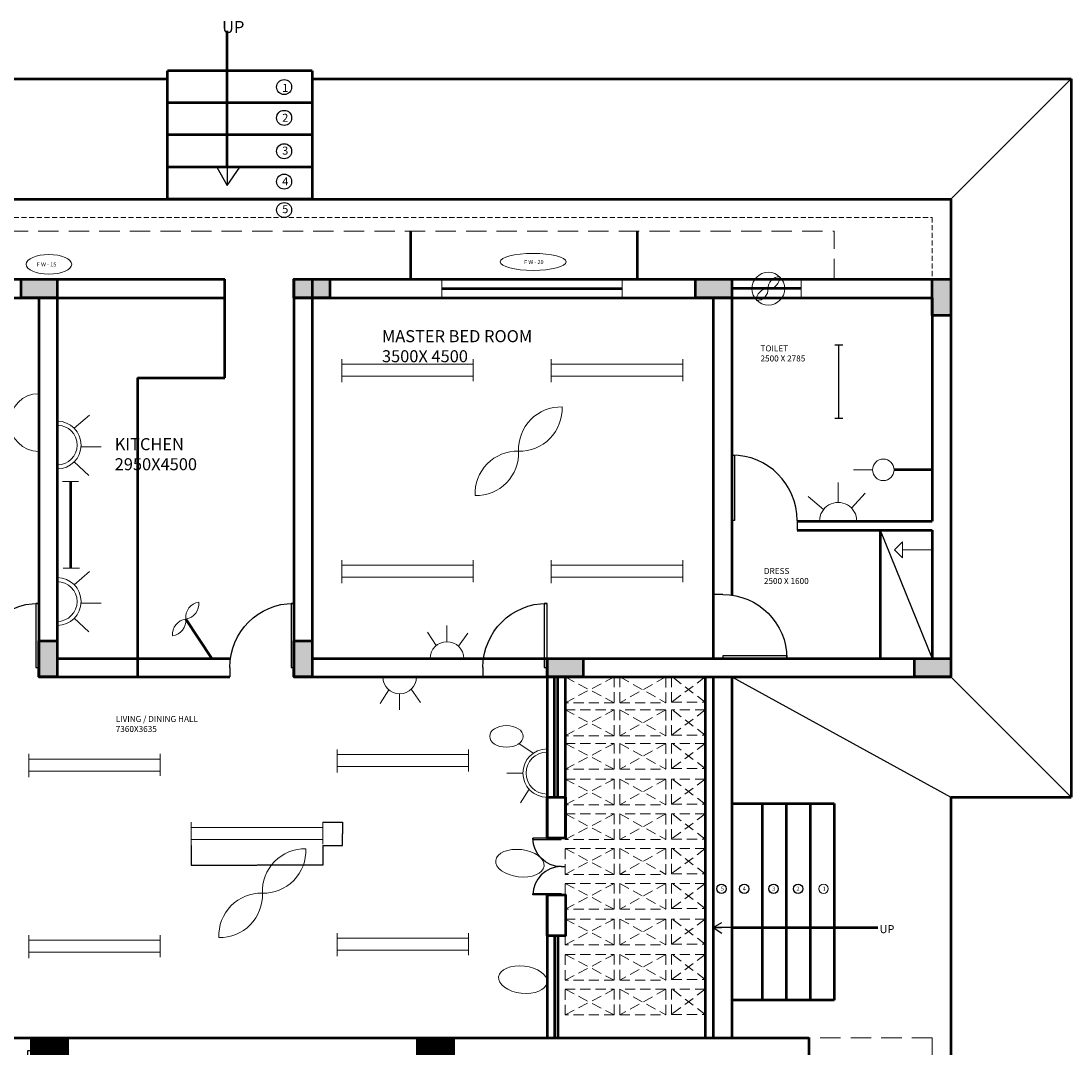
# Model space of a CAD drawing. Units: millimetres. Extents: x 15 to 330868, y -4710 to 1734924.
# Tile 3 of 3: x 317776 to 330868, y 856654 to 869450. Entities that reach past the tile are written whole.
import ezdxf

# ---------------------------------------------------------------- set-up
doc = ezdxf.new("R2010")
doc.units = ezdxf.units.MM
doc.header["$MEASUREMENT"] = 0
doc.linetypes.add('DASHED', pattern=[19.049999999999997, 12.7, -6.349999999999999])
for name, color, linetype, lineweight in [('A-ANNO-DIMS', 2, 'Continuous', 18), ('A-ANNO-TEXT', 7, 'Continuous', 18), ('A-AREA-IDEN', 30, 'Continuous', 25), ('A-COLS', 8, 'Continuous', 35), ('A-DOOR', 4, 'Continuous', 25), ('A-FLOR-OVHD', 8, 'DASHED', 18), ('A-FLOR-STRS', 3, 'Continuous', 25), ('A-ROOF', 6, 'Continuous', 25), ('A-ROOF-OVHD', 6, 'DASHED', 18), ('A-WALL', 7, 'Continuous', 50), ('E-LITE', 1, 'Continuous', 18)]:
    doc.layers.add(name, color=color, linetype=linetype, lineweight=lineweight)
doc.styles.get("Standard").update_dxf_attribs({"font": 'arial.ttf'})
doc.dimstyles.get("Standard").update_dxf_attribs({"dimtxt": 0.18, "dimasz": 0.18, "dimexe": 0.18, "dimexo": 0.0625, "dimgap": 0.09, "dimtad": 0, "dimtih": 1, "dimtoh": 1, "dimdec": 0, "dimzin": 0, "dimdsep": 46, "dimtxsty": 'Standard', "dimcen": 0.09, "dimadec": 0, "dimazin": 0, "dimtfac": 1, "dimtdec": 0, "dimtofl": 0, "dimtmove": 0, "dimatfit": 3, "dimfxl": 1, "dimtolj": 1, "dimtzin": 0, "dimarcsym": 0})

# ---------------------------------------------------------------- blocks, each defined once
blk = doc.blocks.new('*U2')
for p, q in [((0, 4), (7e-16, 0)), ((7e-16, 2), (36, 2)), ((36, 3.999999999999999), (36, -4e-16))]:
    blk.add_line(p, q)
blk = doc.blocks.new('*U5')
for p, q in [((0, 0), (-1e-16, -5.999999999999999)), ((40, -6e-16), (40, -6))]:
    blk.add_line(p, q)
blk.add_lwpolyline([(0, 0), (5.6e-15, 40), (1.750000000000007, 40), (1.749999999999998, -7e-16)], close=True)
blk.add_arc((0, 0), 40, 0, 90)
blk = doc.blocks.new('FAN-CEILING')
blk.add_line((543.2829999999958, 553.5), (543.2829999999958, 553.5))
for centre, radius, start, end in [((555.3863884535967, 1083.047616258962), 529.6859162592511, 268.5279151991481, 2.595751645517247), ((1072.491430036316, 575.9857168442104), 529.6859162592514, 88.52791519914813, 182.5957516455172), ((529.6754217544221, 23.98890125169419), 529.6859162592514, 88.52791519914813, 182.5957516455172), ((14.1405782456859, 529.5110987483058), 529.6859162592514, 268.5279151991481, 2.595751645517247)]:
    blk.add_arc(centre, radius, start, end)
blk = doc.blocks.new('FAN-EXHAUST')
blk.add_line((145.1339548087562, 148.0080506636295), (145.1339548087562, 148.0080506636295))
for centre, radius, start, end in [((148.3704525375506, 289.6113433190621), 141.6402746656115, 268.5279151991481, 2.595751652180509), ((286.6465476204758, 154.0208273150492), 141.6402746656116, 88.52791519914813, 182.5957516521805), ((141.4952303098398, 6.414522946579381), 141.6402746656116, 88.52791519914813, 182.5957516521805), ((3.639012893370818, 141.5933160863351), 141.6402746656116, 268.5279151991481, 2.595751652180509)]:
    blk.add_arc(centre, radius, start, end)
blk = doc.blocks.new('LIGHT-FTL')
for p, q in [((0, 289), (0, 0)), ((1640, 289), (1640, 15)), ((0, 224.5), (1640, 224.5)), ((0, 74.5), (1640, 74.5))]:
    blk.add_line(p, q)
blk = doc.blocks.new('*D11')
at = {"layer": 'A-ANNO-DIMS', "color": 0, "lineweight": -2, "transparency": 16777216}
for p, q in [((319898.5, 859167.4375000001), (319898.5, 858921.3200000001)), ((321538.5, 859167.4375000001), (321538.5, 858921.3200000001)), ((319898.68, 858921.5000000001), (320716.0906889495, 858921.5000000001)), ((321538.32, 858921.5000000001), (320720.9093110505, 858921.5000000001))]:
    blk.add_line(p, q, dxfattribs=at)
at = {"layer": 'A-ANNO-DIMS', "color": 0, "transparency": 16777216}
for points in [[(319898.68, 858921.5300000001), (319898.68, 858921.4699999999), (319898.5, 858921.5000000001)], [(321538.32, 858921.5300000001), (321538.32, 858921.4699999999), (321538.5, 858921.5000000001)]]:
    blk.add_solid(points, dxfattribs=at)
at = {"layer": 'Defpoints', "color": 0, "transparency": 16777216}
for p in [(319898.5, 859167.5), (321538.5, 859167.5), (321538.5, 858921.5000000001)]:
    blk.add_point(p, dxfattribs=at)
at = {"layer": 'A-ANNO-DIMS', "color": 0, "transparency": 16777216, "insert": (320718.5000000001, 858921.5000000001), "char_height": 0.18, "attachment_point": 5}
blk.add_mtext('\\A1;FLUORESCENT TUBE LIGHT 1640 TYP.', dxfattribs=at)
blk = doc.blocks.new('*D12')
at = {"layer": 'A-ANNO-DIMS', "color": 0, "lineweight": -2, "transparency": 16777216}
for p, q in [((321538.5625000001, 859456.5000000006), (321784.6800000002, 859456.5000000006)), ((321784.5000000003, 859456.3200000004), (321784.5000000003, 859312.1819031383)), ((321784.5000000003, 859167.6800000007), (321784.5000000003, 859311.8180968628)), ((321538.5625000001, 859167.5000000005), (321784.6800000002, 859167.5000000005))]:
    blk.add_line(p, q, dxfattribs=at)
at = {"layer": 'A-ANNO-DIMS', "color": 0, "transparency": 16777216}
for points in [[(321784.4700000002, 859456.3200000004), (321784.5300000003, 859456.3200000004), (321784.5000000003, 859456.5000000006)], [(321784.4700000002, 859167.6800000007), (321784.5300000003, 859167.6800000007), (321784.5000000003, 859167.5000000005)]]:
    blk.add_solid(points, dxfattribs=at)
at = {"layer": 'Defpoints', "color": 0, "transparency": 16777216}
for p in [(321538.5000000001, 859456.5000000006), (321784.5000000003, 859456.5000000006), (321538.5000000001, 859167.5000000005)]:
    blk.add_point(p, dxfattribs=at)
at = {"layer": 'A-ANNO-DIMS', "color": 0, "transparency": 16777216, "insert": (321784.5000000004, 859312.0000000002), "char_height": 0.18, "attachment_point": 5}
blk.add_mtext('\\A1;289 TYP.', dxfattribs=at)

msp = doc.modelspace()

# ---------------------------------------------------------------- hatches: boundary and pattern name
at = {"layer": 'A-COLS'}
h = msp.add_hatch(color=256, dxfattribs=at)
h.dxf.hatch_style = 1
h.paths.add_polyline_path([(312687.5462042676, 861499.2884389247), (312237.5462042676, 861499.2884389247), (312237.5462042676, 861269.2884389245), (312687.5462042676, 861269.2884389245)])
h.paths.add_polyline_path([(312687.5462042676, 865999.2884389245), (312687.5462042676, 866229.2884389247), (312237.5462042676, 866229.2884389247), (312237.5462042676, 865999.2884389245)])
h.paths.add_polyline_path([(318227.5462042675, 866229.2884389248), (317777.5462042676, 866229.2884389248), (317777.5462042676, 865999.2884389247), (318227.5462042675, 865999.2884389247)])
h.paths.add_polyline_path([(321177.5462042676, 866229.2884389248), (321177.5462042676, 865999.2884389247), (321627.5462042676, 865999.2884389247), (321627.5462042676, 866229.2884389248)])
h.paths.add_polyline_path([(326187.5462042675, 866229.2884389248), (326187.5462042675, 865999.2884389247), (326637.5462042675, 865999.2884389247), (326637.5462042675, 866229.2884389248)])
h = msp.add_hatch(color=256, dxfattribs=at)
h.dxf.hatch_style = 1
h.paths.add_polyline_path([(329137.5462042676, 865779.2884389246), (329367.5462042676, 865779.2884389246), (329367.5462042676, 866229.2884389247), (329137.5462042676, 866229.2884389247)])
h = msp.add_hatch(color=256, dxfattribs=at)
h.dxf.hatch_style = 1
h.paths.add_polyline_path([(318227.5462042675, 861719.2884389245), (317997.5462042675, 861719.2884389245), (317997.5462042675, 861269.2884389245), (318227.5462042675, 861269.2884389245)])
h.paths.add_polyline_path([(321407.5462042675, 861719.2884389247), (321177.5462042676, 861719.2884389247), (321177.5462042676, 861269.2884389247), (321407.5462042675, 861269.2884389247)])
h = msp.add_hatch(color=256, dxfattribs=at)
h.dxf.hatch_style = 1
h.paths.add_polyline_path([(324334.2049794545, 861499.2884389244), (324334.2049794545, 861269.2884389245), (324784.2049794545, 861269.2884389245), (324784.2049794545, 861499.2884389244)])
h = msp.add_hatch(color=256, dxfattribs=at)
h.dxf.hatch_style = 1
h.paths.add_polyline_path([(329367.5462042676, 861499.2884389247), (328917.5462042675, 861499.2884389247), (328917.5462042675, 861269.2884389247), (329367.5462042676, 861269.2884389247)])
h = msp.add_hatch(dxfattribs=at)
h.set_pattern_fill('ANSI31', color=256, scale=10)
h.set_pattern_definition([(45, (318145, 856621), (-0.8838834764831844, 0.8838834764831844), [])])
h.paths.add_polyline_path([(318357.5, 856769.2884389247), (317907.5, 856769.2884389247), (317907.5, 856539.2884389245), (318357.5, 856539.2884389245)])
h.paths.add_polyline_path([(323167.5, 856769.2884389247), (322717.5000000001, 856769.2884389247), (322717.5000000001, 856539.2884389247), (323167.5, 856539.2884389247)])

# ---------------------------------------------------------------- linework, layer by layer
at = {"layer": 'A-FLOR-OVHD', "ltscale": 10}
for p, q in [((324559.2049794545, 861269.2884389245), (325173, 860948)), ((324559.2049794545, 860948), (325173, 861269.2884389245)), ((325242, 861269.2884389245), (325815, 860948)), ((325815, 861269.2884389245), (325242, 860948)), ((326307.5462042676, 861269.2884389245), (325887.5000000001, 860955)), ((325906, 861261), (326307.5462042676, 860955)), ((324559.2049794545, 860857.9999999998), (325173, 860536.7115610754)), ((324559.2049794545, 860536.7115610754), (325173, 860857.9999999998)), ((325242, 860857.9999999999), (325815, 860536.7115610754)), ((325815, 860857.9999999999), (325242, 860536.7115610754)), ((326307.5462042676, 860857.9999999999), (325887.5000000001, 860543.7115610754)), ((325906, 860849.7115610754), (326307.5462042676, 860543.7115610754)), ((324559.2049794545, 860440.4999999999), (325173, 860119.2115610755)), ((324559.2049794545, 860119.2115610755), (325173, 860440.4999999999)), ((325242, 860440.4999999999), (325815, 860119.2115610755)), ((325815, 860440.4999999999), (325242, 860119.2115610755)), ((326307.5462042676, 860440.4999999999), (325887.5000000001, 860126.2115610756)), ((325906, 860432.2115610756), (326307.5462042676, 860126.2115610756)), ((324559.2049794545, 859995.9999999999), (325173, 859674.7115610755)), ((324559.2049794545, 859674.7115610755), (325173, 859995.9999999999)), ((325242, 859995.9999999999), (325815, 859674.7115610755)), ((325815, 859995.9999999999), (325242, 859674.7115610755)), ((326307.5462042676, 859995.9999999999), (325887.5000000001, 859681.7115610754)), ((325906, 859987.7115610755), (326307.5462042676, 859681.7115610754)), ((324559.2049794545, 859561.4999999998), (325173, 859240.2115610754)), ((324559.2049794545, 859240.2115610754), (325173, 859561.4999999998)), ((325242, 859561.5), (325815, 859240.2115610754)), ((325815, 859561.5), (325242, 859240.2115610754)), ((326307.5462042676, 859561.5), (325887.5000000001, 859247.2115610755)), ((325906, 859553.2115610755), (326307.5462042676, 859247.2115610755)), ((324559.2049794545, 859128.9999999998), (325173, 858807.7115610754)), ((324559.2049794545, 858807.7115610754), (325173, 859128.9999999998)), ((325242, 859128.9999999998), (325815, 858807.7115610754)), ((325815, 859128.9999999998), (325242, 858807.7115610754)), ((326307.5462042676, 859128.9999999998), (325887.5000000001, 858814.7115610755)), ((325906, 859120.7115610755), (326307.5462042676, 858814.7115610755)), ((324559.2049794545, 858693.9999999998), (325173, 858372.7115610754)), ((324559.2049794545, 858372.7115610754), (325173, 858693.9999999998)), ((325242, 858694), (325815, 858372.7115610754)), ((325815, 858694), (325242, 858372.7115610754)), ((326307.5462042676, 858694), (325887.5000000001, 858379.7115610755)), ((325906, 858685.7115610754), (326307.5462042676, 858379.7115610755)), ((324559.2049794545, 858250.4999999997), (325173, 857929.2115610753)), ((324559.2049794545, 857929.2115610753), (325173, 858250.4999999997)), ((325242, 858250.4999999999), (325815, 857929.2115610753)), ((325815, 858250.4999999999), (325242, 857929.2115610753)), ((326307.5462042676, 858250.4999999999), (325887.5000000001, 857936.2115610754)), ((325906, 858242.2115610754), (326307.5462042676, 857936.2115610754)), ((324559.2049794545, 857808.4999999999), (325173, 857487.2115610755)), ((324559.2049794545, 857487.2115610755), (325173, 857808.4999999999)), ((325242, 857808.4999999999), (325815, 857487.2115610755)), ((325815, 857808.4999999999), (325242, 857487.2115610755)), ((326307.5462042676, 857808.4999999999), (325887.5000000001, 857494.2115610754)), ((325906, 857800.2115610756), (326307.5462042676, 857494.2115610754)), ((324559.2049794545, 857374.9999999998), (325173, 857053.7115610754)), ((324559.2049794545, 857053.7115610754), (325173, 857374.9999999998)), ((325242, 857375), (325815, 857053.7115610754)), ((325815, 857375), (325242, 857053.7115610754)), ((326307.5462042676, 857375), (325887.5000000001, 857060.7115610753)), ((325906, 857366.7115610755), (326307.5462042676, 857060.7115610753))]:
    msp.add_line(p, q, dxfattribs=at)
for points in [[(324559.2049794545, 861269.2884389245), (325173, 861269.2884389245), (325173, 860948), (324559.2049794545, 860948)], [(325815, 861269.2884389245), (325242, 861269.2884389245), (325242, 860948), (325815, 860948)], [(326307.5462042676, 861269.2884389245), (325887.5000000001, 861269.2884389245), (325887.5000000001, 860955), (326307.5462042676, 860955)], [(324559.2049794545, 860857.9999999998), (325173, 860857.9999999998), (325173, 860536.7115610754), (324559.2049794545, 860536.7115610754)], [(325815, 860857.9999999999), (325242, 860857.9999999999), (325242, 860536.7115610754), (325815, 860536.7115610754)], [(326307.5462042676, 860857.9999999999), (325887.5000000001, 860857.9999999999), (325887.5000000001, 860543.7115610754), (326307.5462042676, 860543.7115610754)], [(324559.2049794545, 860440.4999999999), (325173, 860440.4999999999), (325173, 860119.2115610755), (324559.2049794545, 860119.2115610755)], [(325815, 860440.4999999999), (325242, 860440.4999999999), (325242, 860119.2115610755), (325815, 860119.2115610755)], [(326307.5462042676, 860440.4999999999), (325887.5000000001, 860440.4999999999), (325887.5000000001, 860126.2115610756), (326307.5462042676, 860126.2115610756)], [(324559.2049794545, 859995.9999999999), (325173, 859995.9999999999), (325173, 859674.7115610755), (324559.2049794545, 859674.7115610755)], [(325815, 859995.9999999999), (325242, 859995.9999999999), (325242, 859674.7115610755), (325815, 859674.7115610755)], [(326307.5462042676, 859995.9999999999), (325887.5000000001, 859995.9999999999), (325887.5000000001, 859681.7115610754), (326307.5462042676, 859681.7115610754)], [(324559.2049794545, 859561.4999999998), (325173, 859561.4999999998), (325173, 859240.2115610754), (324559.2049794545, 859240.2115610754)], [(325815, 859561.5), (325242, 859561.5), (325242, 859240.2115610754), (325815, 859240.2115610754)], [(326307.5462042676, 859561.5), (325887.5000000001, 859561.5), (325887.5000000001, 859247.2115610755), (326307.5462042676, 859247.2115610755)], [(324559.2049794545, 859128.9999999998), (325173, 859128.9999999998), (325173, 858807.7115610754), (324559.2049794545, 858807.7115610754)], [(325815, 859128.9999999998), (325242, 859128.9999999998), (325242, 858807.7115610754), (325815, 858807.7115610754)], [(326307.5462042676, 859128.9999999998), (325887.5000000001, 859128.9999999998), (325887.5000000001, 858814.7115610755), (326307.5462042676, 858814.7115610755)], [(324559.2049794545, 858693.9999999998), (325173, 858693.9999999998), (325173, 858372.7115610754), (324559.2049794545, 858372.7115610754)], [(325815, 858694), (325242, 858694), (325242, 858372.7115610754), (325815, 858372.7115610754)], [(326307.5462042676, 858694), (325887.5000000001, 858694), (325887.5000000001, 858379.7115610755), (326307.5462042676, 858379.7115610755)], [(324559.2049794545, 858250.4999999997), (325173, 858250.4999999997), (325173, 857929.2115610753), (324559.2049794545, 857929.2115610753)], [(325815, 858250.4999999999), (325242, 858250.4999999999), (325242, 857929.2115610753), (325815, 857929.2115610753)], [(326307.5462042676, 858250.4999999999), (325887.5000000001, 858250.4999999999), (325887.5000000001, 857936.2115610754), (326307.5462042676, 857936.2115610754)], [(324559.2049794545, 857808.4999999999), (325173, 857808.4999999999), (325173, 857487.2115610755), (324559.2049794545, 857487.2115610755)], [(325815, 857808.4999999999), (325242, 857808.4999999999), (325242, 857487.2115610755), (325815, 857487.2115610755)], [(326307.5462042676, 857808.4999999999), (325887.5000000001, 857808.4999999999), (325887.5000000001, 857494.2115610754), (326307.5462042676, 857494.2115610754)], [(324559.2049794545, 857374.9999999998), (325173, 857374.9999999998), (325173, 857053.7115610754), (324559.2049794545, 857053.7115610754)], [(325815, 857375), (325242, 857375), (325242, 857053.7115610754), (325815, 857053.7115610754)], [(326307.5462042676, 857375), (325887.5000000001, 857375), (325887.5000000001, 857060.7115610753), (326307.5462042676, 857060.7115610753)]]:
    msp.add_lwpolyline(points, close=True, dxfattribs=at)
at = {"layer": 'A-FLOR-STRS'}
for p, q in [((320504.5000000001, 867629.2884389248), (320218.5, 867629.2884389248)), ((320218.5, 867629.2884389248), (320345, 867397.5)), ((320345, 867629.2884389248), (320345, 867397.5)), ((320345, 867397.5), (320504.5000000001, 867629.2884389248)), ((326407.5462042676, 858143.5), (326516, 858205.5)), ((326637.5462042676, 858143.5), (326407.5462042676, 858143.5)), ((326407.5462042676, 858143.5), (326510, 858143.5)), ((326407.5462042676, 858143.5), (326513.5, 858075.5000000001)), ((326637.5462042676, 857239.5), (326637.5462042676, 857239.5))]:
    msp.add_line(p, q, dxfattribs=at)
for centre, radius in [((321057, 868626), 93.49999999999999), ((321057, 868242), 93.49999999999999), ((321057, 867826), 93.49999999999999), ((321057, 867447), 93.49999999999999), ((321057, 867092.7884389248), 93.49999999999999), ((326510, 858628), 58), ((326793.5, 858628), 58), ((327159, 858628), 58), ((327465.5, 858628), 58)]:
    msp.add_circle(centre, radius, dxfattribs=at)
at = {"layer": 'A-ROOF'}
for p, q in [((329367.5462042676, 867229.2884389248), (330867.5462042675, 868729.2884389249)), ((328489.5000000001, 863099.2884389248), (329137.5462042676, 861499.2884389247)), ((326637.5462042676, 861269.2884389245), (329367.5462042676, 859769.2884389244)), ((329367.5462042676, 861269.2884389247), (330867.5462042675, 859769.2884389246))]:
    msp.add_line(p, q, dxfattribs=at)
at = {"layer": 'A-ROOF-OVHD', "ltscale": 5}
for p, q in [((313305.0000000001, 866999.288438925), (329137.5462042676, 866999.2884389248)), ((329137.5462042676, 866999.2884389248), (329137.5462042676, 866229.2884389248))]:
    msp.add_line(p, q, dxfattribs=at)
at = {"layer": 'A-ROOF-OVHD', "ltscale": 20}
for p, q in [((313418.5, 866829.2884389249), (327915, 866829.2884389247)), ((327915, 866229.2884389248), (327915, 866829.2884389247)), ((329137.5462042676, 856769.2884389244), (327597.5000000001, 856769.2884389244)), ((329137.5462042676, 856769.2884389244), (329137.5462042676, 848959.2884389248))]:
    msp.add_line(p, q, dxfattribs=at)
at = {"layer": 'A-WALL'}
for p, q in [((320345, 867629.2884389248), (320345, 869326.5000000002)), ((309737.5462042676, 868729.2884389249), (319602.7731021338, 868729.2884389249)), ((321406.2268978663, 868729.2884389249), (330867.5462042675, 868729.2884389249)), ((330867.5462042675, 868729.2884389249), (330867.5462042675, 867729.2884389247)), ((330867.5462042675, 867729.2884389247), (330867.5462042675, 859769.2884389244)), ((311237.5462042676, 867229.2884389248), (329367.5462042676, 867229.2884389248)), ((329367.5462042675, 867229.2884389248), (329367.5462042675, 861269.2884389247)), ((322636.5, 866229.2884389247), (322636.5, 866829.2884389247)), ((325461, 866229.2884389247), (325461, 866829.2884389247)), ((314267.5462042676, 866229.2884389247), (320317.5462042675, 866229.2884389248)), ((318227.5462042675, 866229.2884389247), (318227.5462042675, 861269.2884389245)), ((320317.5462042676, 864999.2884389247), (320317.5462042676, 866229.2884389248)), ((321177.5462042676, 866229.2884389247), (321177.5462042676, 861269.2884389247)), ((321177.5462042676, 866229.2884389247), (329367.5462042676, 866229.2884389248)), ((321407.5462042675, 866229.2884389247), (321407.5462042675, 861269.2884389245)), ((326637.5462042676, 866229.2884389247), (326637.5462042676, 862289.9804837471)), ((323021.5000000001, 866114.2884389247), (325272.5462042675, 866114.2884389247)), ((327501.5000000001, 866114.2884389247), (326637.5462042675, 866114.2884389247)), ((314497.5462042676, 865999.2884389247), (320317.5462042676, 865999.2884389248)), ((317997.5462042676, 865999.288438925), (317997.5462042676, 861269.2884389245)), ((321177.5462042676, 865999.288438925), (329137.5462042676, 865999.2884389248)), ((326407.5462042676, 865999.2884389252), (326407.5462042676, 861499.2884389247)), ((329137.5462042676, 865999.2884389248), (329137.5462042676, 863214.2884389249)), ((319227.5462042676, 864999.2884389247), (320317.5462042676, 864999.2884389247)), ((319227.5462042676, 864999.2884389247), (319227.5462042676, 861269.2884389245)), ((329137.5462042676, 863852.4999999999), (328661.5000000001, 863852.4999999999)), ((318393, 863709), (318393, 862628)), ((327452.9332805257, 863214.2884389248), (329137.5462042676, 863214.2884389249)), ((327452.9332805257, 863099.2884389247), (329137.5462042676, 863099.2884389248)), ((328489.5000000001, 863099.2884389248), (328489.5000000001, 861499.2884389247)), ((329137.5462042676, 863099.2884389248), (329137.5462042676, 861499.2884389247)), ((320154, 861499.2884389247), (319830.5, 861992)), ((318227.5462042675, 861499.2884389247), (320386.8541594451, 861499.2884389245)), ((321407.5462042675, 861499.2884389247), (324796.8541594452, 861499.2884389248)), ((324334.2049794545, 861499.2884389247), (324334.2049794545, 859257.053530784)), ((324784.2049794545, 861499.2884389247), (329367.5462042676, 861499.2884389247)), ((317997.5462042676, 861269.2884389245), (320379.2049794545, 861269.2884389245)), ((321177.5462042676, 861269.2884389245), (324789.2049794544, 861269.2884389247)), ((324429.5563246001, 859768.7936142335), (324429.5563246001, 861269.2884389245)), ((324469.5563246001, 859768.7936142335), (324469.5563246001, 861269.2884389245)), ((324559.2049794545, 861269.2884389245), (324559.2049794545, 859257.053530784)), ((324784.2049794545, 861269.2884389245), (329367.5462042676, 861269.2884389247)), ((326307.5462042676, 861269.2884389245), (326307.5462042676, 856769.2884389247)), ((326407.5462042676, 861269.2884389245), (326407.5462042676, 856769.2884389247)), ((326637.5462042676, 861269.2884389245), (326637.5462042676, 856769.2884389247)), ((329367.5462042676, 859769.2884389244), (330867.5462042675, 859769.2884389246)), ((329367.5462042676, 859769.2884389244), (329367.5462042677, 851619.2884389246)), ((326637.5462042676, 859691.0000000001), (327915.5924085352, 859691.0000000001)), ((327015.5924085351, 859691.0000000001), (327015.5924085351, 857239.5)), ((327315.5924085351, 859691.0000000001), (327315.5924085351, 857239.5)), ((327615.5924085351, 859691.0000000001), (327615.5924085351, 857239.5)), ((327915.5924085352, 859691.0000000001), (327915.5924085352, 857239.5)), ((324334.2049794545, 858551.5233470649), (324334.2049794545, 856769.2884389247)), ((324429.5563246001, 858039.7832636154), (324429.5563246001, 856769.2884389247)), ((324469.5563246001, 858039.7832636154), (324469.5563246001, 856769.2884389247)), ((326637.5462042676, 858143.5), (328461, 858143.5)), ((327915.5924085352, 857239.5), (326637.5462042676, 857239.5)), ((313477.5, 856769.2884389245), (321177.5462042676, 856769.2884389247)), ((321177.5462042677, 856769.2884389247), (327597.5000000001, 856769.2884389244)), ((327597.5000000001, 856769.2884389245), (327597.5000000001, 855942.5))]:
    msp.add_line(p, q, dxfattribs=at)
for points in [[(321406.2268978663, 868829.2884389246), (321406.2268978663, 867229.2884389248), (319602.7731021338, 867229.2884389248), (319602.7731021338, 868829.2884389246)], [(321406.2268978663, 868829.2884389246), (319602.7731021338, 868829.2884389246)], [(321406.2268978663, 868429.2884389249), (319602.7731021338, 868429.2884389249)], [(321406.2268978663, 868029.2884389247), (319602.7731021338, 868029.2884389247)], [(321406.2268978663, 867629.2884389248), (319602.7731021338, 867629.2884389248)], [(329137.5462042676, 866229.2884389247), (329367.5462042676, 866229.2884389247), (329367.5462042676, 865779.2884389246), (329137.5462042676, 865779.2884389246), (329137.5462042676, 866229.2884389247)]]:
    msp.add_lwpolyline(points, dxfattribs=at)
for points in [[(318227.5462042675, 866229.2884389248), (318227.5462042675, 865999.2884389247), (317777.5462042676, 865999.2884389247), (317777.5462042676, 866229.2884389248)], [(321627.5462042676, 866229.2884389248), (321627.5462042676, 865999.2884389247), (321177.5462042676, 865999.2884389247), (321177.5462042676, 866229.2884389248)], [(326637.5462042675, 866229.2884389248), (326637.5462042675, 865999.2884389247), (326187.5462042675, 865999.2884389247), (326187.5462042675, 866229.2884389248)], [(317997.5462042675, 861719.2884389245), (318227.5462042675, 861719.2884389245), (318227.5462042675, 861269.2884389245), (317997.5462042675, 861269.2884389245)], [(321177.5462042676, 861719.2884389247), (321407.5462042675, 861719.2884389247), (321407.5462042675, 861269.2884389247), (321177.5462042676, 861269.2884389247)], [(324784.2049794545, 861499.2884389244), (324784.2049794545, 861269.2884389245), (324334.2049794545, 861269.2884389245), (324334.2049794545, 861499.2884389244)], [(329367.5462042676, 861499.2884389247), (329367.5462042676, 861269.2884389247), (328917.5462042675, 861269.2884389247), (328917.5462042675, 861499.2884389247)], [(324334.9076697458, 859768.7936142335), (324564.2049794545, 859768.7936142335), (324564.2049794545, 859257.053530784), (324334.9076697458, 859257.053530784)], [(324334.9076697458, 858551.5233470649), (324564.2049794545, 858551.5233470649), (324564.2049794545, 858039.7832636154), (324334.9076697458, 858039.7832636154)], [(318357.5, 856769.2884389247), (318357.5, 856539.2884389245), (317907.5, 856539.2884389245), (317907.5, 856769.2884389247)], [(323167.5, 856769.2884389247), (323167.5, 856539.2884389247), (322717.5000000001, 856539.2884389247), (322717.5000000001, 856769.2884389247)]]:
    msp.add_lwpolyline(points, close=True, dxfattribs=at)
at = {"layer": 'E-LITE'}
for p, q in [((323021.5000000001, 866229.2884389248), (323021.5000000001, 865999.288438925)), ((325272.5462042675, 866229.2884389247), (325272.5462042675, 865999.288438925)), ((327501.5000000001, 866229.2884389248), (327501.5000000001, 865999.2884389248)), ((318439.051171271, 864371.5473728542), (318628.5408834528, 864534.6229656857)), ((318439.051171271, 864371.5473728542), (318439.051171271, 864371.5473728542)), ((318524.8496627311, 864139.9383791034), (318774.8496627311, 864139.9383791034)), ((318440.7435920348, 863953.1706363488), (318623.2758062252, 863782.3432650561)), ((328393.5, 863852.4999999999), (328157, 863852.4999999999)), ((318293, 863709), (318493, 863709)), ((327964.5, 863446.2954431295), (327964.5, 863696.2954431295)), ((328131.4767118364, 863375.3661459619), (328299.7179404539, 863560.2847469551)), ((327781.7904987702, 863357.2726623915), (327590.833940531, 863518.6281484013)), ((328666.5, 862854.9999999998), (328766.5, 862954.9999999998)), ((328766.5, 862854.9999999998), (328766.5, 862954.9999999998)), ((328766.5, 862754.9999999997), (328666.5, 862854.9999999998)), ((329137.5462042676, 862854.9999999998), (328766.5, 862854.9999999998)), ((328766.5, 862854.9999999998), (328766.5, 862754.9999999997)), ((318302, 862628), (318506, 862628)), ((318439.051171271, 862420.1915923165), (318628.5408834528, 862583.267185148)), ((318439.051171271, 862420.1915923165), (318439.051171271, 862420.1915923165)), ((318524.8496627311, 862188.5825985655), (318774.8496627311, 862188.5825985655)), ((318440.7435920348, 862001.8148558111), (318623.2758062252, 861830.9874845186)), ((322951.4617291272, 861660.1133915898), (322845.2806171569, 861829.5995900272)), ((323086.5, 861709.2884389249), (323086.5, 861909.288438925)), ((323229.5678242209, 861653.014161147), (323345.3641397665, 861816.0822858865)), ((322361.9617291272, 861108.4634862598), (322255.7806171569, 860938.9772878223)), ((322497, 861059.2884389246), (322497, 860859.2884389247)), ((322640.0678242209, 861115.5627167027), (322755.8641397665, 860952.4945919631)), ((324162.3044808791, 860317.5291597272), (323984.8142508988, 860438.4471772249)), ((324033.2511837219, 860070.5000000001), (323833.2511837219, 860070.5000000001)), ((324110.5610105869, 859869.1134007564), (324003.2015613564, 859700.3711456422)), ((324564.2049794545, 858904.2884389245), (324511.2902156755, 858904.2884389245))]:
    msp.add_line(p, q, dxfattribs=at)
for centre, radius in [((327094.1289998794, 866112.1786762056), 204.7952742509166), ((328527.5, 863852.4999999999), 134), ((327782, 858628), 58)]:
    msp.add_circle(centre, radius, dxfattribs=at)
for centre, radius, start, end in [((317997.5462042676, 864442), 360.0402755247991, 90, 270), ((318227.5462042675, 864161.4999999999), 298.0843000060212, 270, 90), ((318227.5462042675, 864161.4999999999), 248.0843000060212, 270, 90), ((327964.5, 863214.2884389249), 232.0070042046722, 359.9999999999712, 180.0000000000287), ((318227.5462042675, 862210.1442194624), 298.0843000060212, 270, 90), ((318227.5462042675, 862210.1442194624), 248.0843000060212, 270, 90), ((320022.1642472075, 862011.9446684332), 192.6991786607235, 98.55456766370558, 185.9408427320273), ((319801.8357527926, 862182.555331567), 192.6991786607235, 278.5545676628192, 5.940842730657482), ((319857.8203409778, 861801.2473527654), 192.6991786607235, 98.15069550896877, 185.5369705889829), ((319638.6999275933, 861973.4068377331), 192.6991786607235, 278.1506955089688, 5.536970588982954), ((323086.5, 861499.2884389248), 210, 0, 180), ((322497, 861269.2884389247), 210, 180, 0), ((324334.2049794545, 860070.5000000001), 300.953795732581, 90, 270), ((324334.2049794545, 860070.5000000001), 260.9537957325811, 90, 270)]:
    msp.add_arc(centre, radius, start, end, dxfattribs=at)
for centre, major_axis, ratio in [((324161.189451064, 866446.5058140534), (411.9999999999999, 0), 0.2572815533980583), ((318124, 866415.5), (284, 0), 0.4294367409771678), ((323828.6694492642, 860528.3023196458), (209.1857491011615, 0.0528227750910446), 0.6456622380973068), ((323996.4184035434, 858946.3821525944), (302.0187231914023, -35.13048136071301), 0.5607537598746313), ((324032.1862562631, 857494.6304813607), (302.0187231914023, -35.13048136071301), 0.5607537598746313)]:
    msp.add_ellipse(centre, major_axis=major_axis, ratio=ratio, dxfattribs=at)

# ---------------------------------------------------------------- block references
at = {"layer": 'A-DOOR'}
for name, p, xscale, yscale, zscale, rotation in [('*U2', (328023.8, 864498.6000000001), 25.4, 25.4, 25.4, 90), ('*U5', (326527.2973879895, 861499.2884389247), -19.95853062032723, 19.95853062032723, 19.95853062032723, 270), ('*U5', (324511.2902156755, 859257.053530784), -8.819127296487046, 8.819127296487046, 8.819127296487046, 90), ('*U5', (324511.2902156755, 858551.5233470649), 8.819127296487046, 8.819127296487046, 8.819127296487046, 90.00000000000003), ('*U5', (317907.5, 856612.6702075743), 26.10303855837779, 26.10303855837779, 26.10303855837779, 180)]:
    msp.add_blockref(name, p, dxfattribs=dict(at, xscale=xscale, yscale=yscale, zscale=zscale, rotation=rotation))
for p, xscale, yscale, zscale in [((326637.5462042676, 863221.5965003636), 20.38467690645148, 20.38467690645148, 20.38467690645148), ((317997.5462042675, 861389.0396226466), -19.95853062032723, 19.95853062032723, 19.95853062032723), ((321177.5462042676, 861389.0396226466), -19.95853062032723, 19.95853062032723, 19.95853062032723), ((324334.2049794545, 861389.0396226464), -19.95853062032723, 19.95853062032723, 19.95853062032723)]:
    msp.add_blockref('*U5', p, dxfattribs=dict(at, xscale=xscale, yscale=yscale, zscale=zscale))
at = {"layer": 'E-LITE'}
for name, p in [('FAN-EXHAUST', (326945.7585473419, 865964.2076075522)), ('LIGHT-FTL', (321775.5, 864945)), ('LIGHT-FTL', (324386, 864945)), ('FAN-CEILING', (323437.1944862228, 863531.9999999998)), ('LIGHT-FTL', (321775.5, 862437.5)), ('LIGHT-FTL', (324386, 862437.5)), ('LIGHT-FTL', (317872.5, 860020)), ('LIGHT-FTL', (321717, 860077)), ('LIGHT-FTL', (319898.5, 859167.5)), ('FAN-CEILING', (320242.3594217545, 858019.674817511)), ('LIGHT-FTL', (317872.5, 857761.4999999999)), ('LIGHT-FTL', (321717, 857786.5))]:
    msp.add_blockref(name, p, dxfattribs=at)

# ---------------------------------------------------------------- texts
at = {"layer": 'A-ANNO-TEXT', "attachment_point": 1}
for s, width, insert, char_height in [('UP', 4478, (320284, 869450.2053206003), 150), ('1', 4478, (321032.5, 868666.5000000001), 100), ('2', 4478, (321032.5, 868292.9092769441), 100), ('3', 4478, (321032.5, 867883.4092769442), 100), ('4', 4478, (321032.5, 867498.9092769441), 100), ('5', 4478, (321032.5, 867152.986154794), 100), ('F W - 15', 696.4999999999999, (317973.5, 866439.5), 50), ('F W - 20', 696.4999999999999, (324048.6894510641, 866468.2445589374), 50), ('5', 4478, (326501.5, 858654.5), 50), ('4', 4478, (326775, 858654.5), 50), ('3', 4478, (327142, 858654.5), 50), ('2', 4478, (327446, 858654.5), 50), ('1', 4478, (327772, 858654.5), 50), ('UP', 4478, (328481, 858174.2046384722), 100)]:
    msp.add_mtext_dynamic_manual_height_columns(s, width=width, gutter_width=1, heights=[0], dxfattribs=dict(at, insert=insert, char_height=char_height))
at = {"layer": 'A-AREA-IDEN', "char_height": 150, "attachment_point": 1}
for s, insert in [('MASTER BED ROOM\\P3500X 4500', (322276.5000000001, 865594.5)), ('{\\H0.5x;TOILET\\P2500 X 2785}', (326996, 865404)), ('KITCHEN \\P2950X4500', (318944.5, 864247.5000000001)), ('{\\H0.5x;DRESS\\P2500 X 1600}', (327038.5, 862628.5000000001)), ('{\\H0.5x;LIVING / DINING HALL\\P7360X3635}', (318957, 860783))]:
    msp.add_mtext_dynamic_manual_height_columns(s, width=7683.453795732522, gutter_width=1, heights=[0], dxfattribs=dict(at, insert=insert))

# ---------------------------------------------------------------- dimensions: what is measured, and where the dimension line sits
at = {"layer": 'A-ANNO-DIMS'}
dim = msp.add_linear_dim(base=(321784.5000000003, 859456.5000000006), p1=(321538.5, 859167.5), p2=(321538.5, 859456.5000000001), angle=90, text='<> TYP.', dimstyle='Standard', override={"dimdec": 0, "dimlfac": 1, "dimrnd": 0, "dimzin": 0, "dimdsep": 46, "dimlunit": 2}, dxfattribs=at)
dim.commit()
dim.dimension.update_dxf_attribs({"geometry": '*D12', "text_midpoint": (321784.5000000004, 859312.0000000002)})
dim = msp.add_linear_dim(base=(321538.5, 858921.5000000001), p1=(319898.5, 859167.5), p2=(321538.5, 859167.5), text='FLUORESCENT TUBE LIGHT <> TYP.', dimstyle='Standard', override={"dimdec": 0, "dimlfac": 1, "dimrnd": 0, "dimzin": 0, "dimdsep": 46, "dimlunit": 2}, dxfattribs=at)
dim.commit()
dim.dimension.update_dxf_attribs({"geometry": '*D11', "text_midpoint": (320718.5000000001, 858921.5000000001)})

doc.saveas('drawing.dxf')
